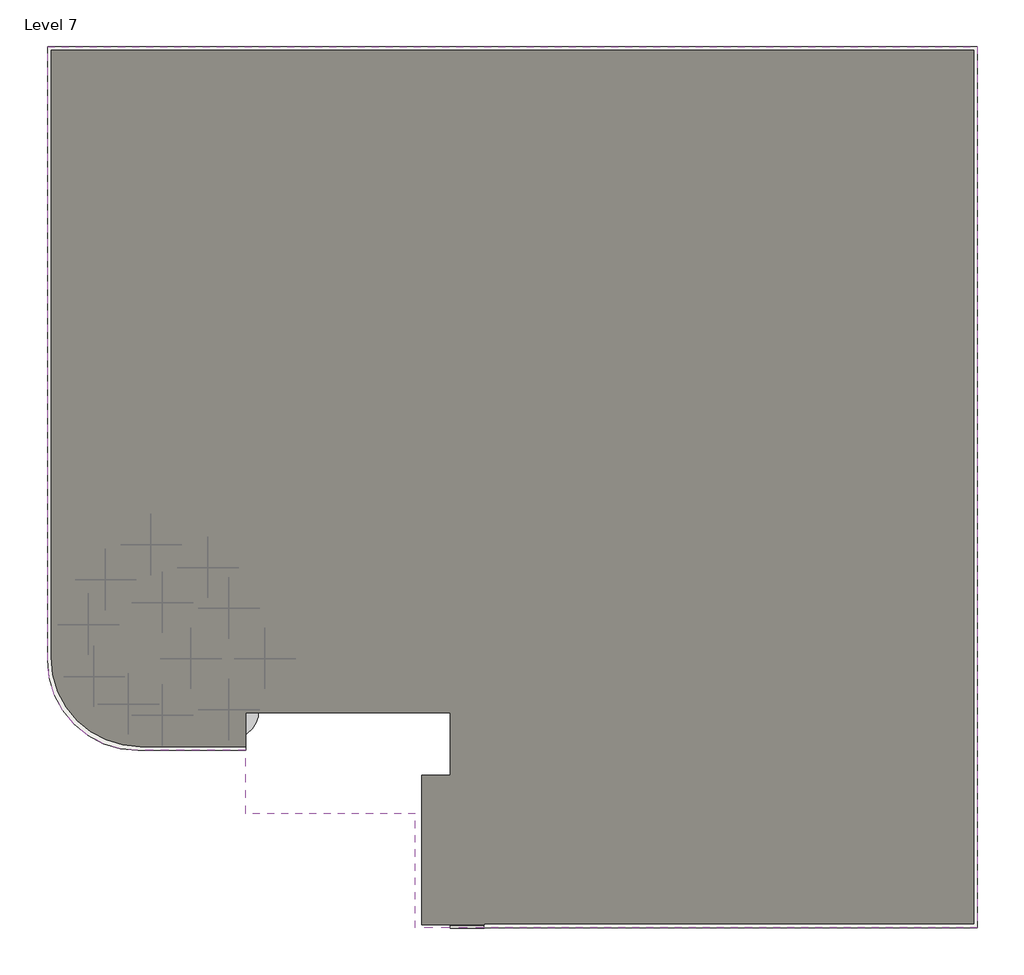
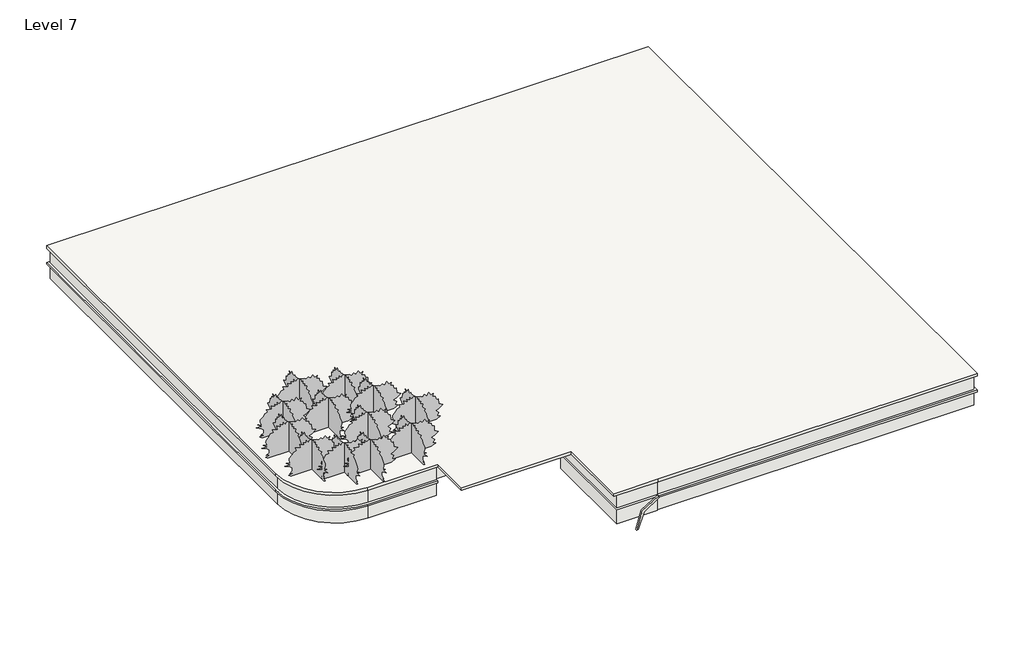
# One storey: 12 geographic elements, 4 slabs, 1 wall.
"""IFC4 building model written with IfcOpenShell, lengths in millimetres."""

from ifc_helpers import new_model, si_unit, point, frame, frame_2d, origin, place, context, project, spatial, polyline, circle_curve, trimmed, segment, composite_curve, outline, extrude, transform, mapped, element, save
from components import rpc_shrub_d2795376

model = new_model("IFC4")

# Units and contexts
model_context = context("Model", 3, world=origin())
ifc_project = project(units=[si_unit("LENGTHUNIT", "METRE", prefix="MILLI")], contexts=[model_context])

# Site, building, storey
site = spatial("IfcSite", under=ifc_project)
building = spatial("IfcBuilding", under=site)
storey = spatial("IfcBuildingStorey", under=building, Name="Level 7", Elevation=15240.0)

# Geographic elements
placement = place(None, origin())
rpc_shrub_shape = rpc_shrub_d2795376(model_context)
element("IfcGeographicElement", 1, ObjectType="RPC Shrub", at=placement, inside=storey, context=model_context, shape_type="MappedRepresentation", body=[
    mapped(rpc_shrub_shape, transform((-13877.236879, -1580.5602909, 16306.8), x_axis=(1.0, 0.0, 0.0), y_axis=(0.0, 1.0, 0.0), z_axis=(0.0, 0.0, 1.0))),
])
element("IfcGeographicElement", 2, ObjectType="RPC Shrub", at=placement, inside=storey, context=model_context, shape_type="MappedRepresentation", body=[
    mapped(rpc_shrub_shape, transform((-11896.036879, -1580.5602909, 16306.8), x_axis=(1.0, 0.0, 0.0), y_axis=(0.0, 1.0, 0.0), z_axis=(0.0, 0.0, 1.0))),
])
element("IfcGeographicElement", 3, ObjectType="RPC Shrub", at=placement, inside=storey, context=model_context, shape_type="MappedRepresentation", body=[
    mapped(rpc_shrub_shape, transform((-14639.236879, -3104.5602909, 16306.8), x_axis=(1.0, 0.0, 0.0), y_axis=(0.0, 1.0, 0.0), z_axis=(0.0, 0.0, 1.0))),
])
element("IfcGeographicElement", 4, ObjectType="RPC Shrub", at=placement, inside=storey, context=model_context, shape_type="MappedRepresentation", body=[
    mapped(rpc_shrub_shape, transform((-16163.236879, 529.4091958, 16306.8), x_axis=(1.0, 0.0, 0.0), y_axis=(0.0, 1.0, 0.0), z_axis=(0.0, 0.0, 1.0))),
])
element("IfcGeographicElement", 5, ObjectType="RPC Shrub", at=placement, inside=storey, context=model_context, shape_type="MappedRepresentation", body=[
    mapped(rpc_shrub_shape, transform((-14639.236879, -80.1908042, 16306.8), x_axis=(1.0, 0.0, 0.0), y_axis=(0.0, 1.0, 0.0), z_axis=(0.0, 0.0, 1.0))),
])
element("IfcGeographicElement", 6, ObjectType="RPC Shrub", at=placement, inside=storey, context=model_context, shape_type="MappedRepresentation", body=[
    mapped(rpc_shrub_shape, transform((-12861.236879, -2952.1602909, 16306.8), x_axis=(1.0, 0.0, 0.0), y_axis=(0.0, 1.0, 0.0), z_axis=(0.0, 0.0, 1.0))),
])
element("IfcGeographicElement", 7, ObjectType="RPC Shrub", at=placement, inside=storey, context=model_context, shape_type="MappedRepresentation", body=[
    mapped(rpc_shrub_shape, transform((-12861.236879, -232.5908042, 16306.8), x_axis=(1.0, 0.0, 0.0), y_axis=(0.0, 1.0, 0.0), z_axis=(0.0, 0.0, 1.0))),
])
element("IfcGeographicElement", 8, ObjectType="RPC Shrub", at=placement, inside=storey, context=model_context, shape_type="MappedRepresentation", body=[
    mapped(rpc_shrub_shape, transform((-16620.436879, -666.1602909, 16306.8), x_axis=(1.0, 0.0, 0.0), y_axis=(0.0, 1.0, 0.0), z_axis=(0.0, 0.0, 1.0))),
])
element("IfcGeographicElement", 9, ObjectType="RPC Shrub", at=placement, inside=storey, context=model_context, shape_type="MappedRepresentation", body=[
    mapped(rpc_shrub_shape, transform((-14944.036879, 1467.4397091, 16306.8), x_axis=(1.0, 0.0, 0.0), y_axis=(0.0, 1.0, 0.0), z_axis=(0.0, 0.0, 1.0))),
])
element("IfcGeographicElement", 10, ObjectType="RPC Shrub", at=placement, inside=storey, context=model_context, shape_type="MappedRepresentation", body=[
    mapped(rpc_shrub_shape, transform((-13420.036879, 857.8397091, 16306.8), x_axis=(1.0, 0.0, 0.0), y_axis=(0.0, 1.0, 0.0), z_axis=(0.0, 0.0, 1.0))),
])
element("IfcGeographicElement", 11, ObjectType="RPC Shrub", at=placement, inside=storey, context=model_context, shape_type="MappedRepresentation", body=[
    mapped(rpc_shrub_shape, transform((-16468.036879, -2061.3908042, 16306.8), x_axis=(1.0, 0.0, 0.0), y_axis=(0.0, 1.0, 0.0), z_axis=(0.0, 0.0, 1.0))),
])
element("IfcGeographicElement", 12, ObjectType="RPC Shrub", at=placement, inside=storey, context=model_context, shape_type="MappedRepresentation", body=[
    mapped(rpc_shrub_shape, transform((-15553.636879, -2799.7602909, 16306.8), x_axis=(1.0, 0.0, 0.0), y_axis=(0.0, 1.0, 0.0), z_axis=(0.0, 0.0, 1.0))),
])

# Slabs
element("IfcSlab", 13, ObjectType="Generic - 2'", at=placement, inside=storey, context=model_context, shape_type="SweptSolid", body=[
    extrude(outline(composite_curve([segment(polyline([(7112.0, -8690.7908042), (-6003.236879, -8690.7908042), (-6003.236879, -8716.1908042), (-7679.636879, -8716.1908042), (-7679.636879, -4704.7602909), (-7374.836879, -4704.7602909), (-6917.636879, -4704.7602909), (-6917.636879, -3028.3602909), (-12404.036879, -3028.3602909), (-12404.036879, -3940.9908042), (-15222.9504174, -3940.9908042)]), True, "CONTINUOUS"), segment(trimmed(circle_curve(frame_2d((-15222.9504174, -1548.7562261)), 2392.2345781), [point((-15222.9504174, -3940.9908042))], [point((-17615.1849955, -1548.7562261))], False, "CARTESIAN"), True, "CONTINUOUS"), segment(polyline([(-17615.1849955, -1548.7562261), (-17615.1849955, 14724.0625), (-6003.236879, 14724.0625), (7112.0, 14724.0625), (7112.0, -8690.7908042)]), True, "CONTINUOUS")], self_intersect=False)), frame((0.0, 0.0, 15163.8), z_axis=(0.0, 0.0, 1.0), x_axis=(1.0, 0.0, 0.0)), (0.0, 0.0, 1.0), 609.6),
])
element("IfcSlab", 14, ObjectType="Generic - 2'", at=placement, inside=storey, context=model_context, shape_type="SweptSolid", body=[
    extrude(outline(composite_curve([segment(polyline([(7112.0, -8690.7908042), (-6003.236879, -8690.7908042), (-6003.236879, -8716.1908042), (-7679.636879, -8716.1908042), (-7679.636879, -4704.7602909), (-7374.836879, -4704.7602909), (-6917.636879, -4704.7602909), (-6917.636879, -3028.3602909), (-12404.036879, -3028.3602909), (-12404.036879, -3940.9908042), (-15222.9504174, -3940.9908042)]), True, "CONTINUOUS"), segment(trimmed(circle_curve(frame_2d((-15222.9504174, -1548.7562261)), 2392.2345781), [point((-15222.9504174, -3940.9908042))], [point((-17615.1849955, -1548.7562261))], False, "CARTESIAN"), True, "CONTINUOUS"), segment(polyline([(-17615.1849955, -1548.7562261), (-17615.1849955, 14724.0625), (-6003.236879, 14724.0625), (7112.0, 14724.0625), (7112.0, -8690.7908042)]), True, "CONTINUOUS")], self_intersect=False)), frame((0.0, 0.0, 15849.6), z_axis=(0.0, 0.0, 1.0), x_axis=(1.0, 0.0, 0.0)), (0.0, 0.0, 1.0), 609.6),
])
element("IfcSlab", 15, ObjectType="Generic - 3\"", at=placement, inside=storey, context=model_context, shape_type="SweptSolid", body=[
    extrude(outline(composite_curve([segment(polyline([(-6003.236879, 14825.6625), (7213.6, 14825.6625), (7213.6, -8792.3908042), (-6003.236879, -8792.3908042), (-6003.236879, -2875.9602909), (-6892.236879, -2875.9602909), (-6915.8673923, -2899.5908042), (-12397.5833185, -2899.5908042), (-12397.5833185, -3051.9908042), (-12397.5833185, -4040.2121743), (-15293.1833185, -4040.2121743)]), True, "CONTINUOUS"), segment(trimmed(circle_curve(frame_2d((-15293.1833185, -1620.7586138)), 2419.4535605), [point((-15293.1833185, -4040.2121743))], [point((-17712.636879, -1620.7586138))], False, "CARTESIAN"), True, "CONTINUOUS"), segment(polyline([(-17712.636879, -1620.7586138), (-17712.636879, 14825.6625), (-6003.236879, 14825.6625)]), True, "CONTINUOUS")], self_intersect=False)), frame((0.0, 0.0, 15773.4), z_axis=(0.0, 0.0, 1.0), x_axis=(1.0, 0.0, 0.0)), (0.0, 0.0, 1.0), 76.2),
])
element("IfcSlab", 16, ObjectType="Generic - 5\"", at=placement, inside=storey, context=model_context, shape_type="SweptSolid", body=[
    extrude(outline(composite_curve([segment(polyline([(-6003.236879, 14825.6625), (7213.6, 14825.6625), (7213.6, -8792.3908042), (-6003.236879, -8792.3908042), (-7850.9833185, -8792.3908042), (-7850.9833185, -5740.4), (-12397.5833185, -5740.4), (-12397.5833185, -4040.2121743), (-15293.1833185, -4040.2121743)]), True, "CONTINUOUS"), segment(trimmed(circle_curve(frame_2d((-15293.1833185, -1620.7586138)), 2419.4535605), [point((-15293.1833185, -4040.2121743))], [point((-17712.636879, -1620.7586138))], False, "CARTESIAN"), True, "CONTINUOUS"), segment(polyline([(-17712.636879, -1620.7586138), (-17712.636879, 14825.6625), (-6003.236879, 14825.6625)]), True, "CONTINUOUS")], self_intersect=False)), frame((0.0, 0.0, 16459.2), z_axis=(0.0, 0.0, 1.0), x_axis=(1.0, 0.0, 0.0)), (0.0, 0.0, 1.0), 127.0),
])

# Wall
element("IfcWall", 17, ObjectType="Generic - 3\"", at=placement, inside=storey, context=model_context, shape_type="SweptSolid", body=[
    extrude(outline(composite_curve([segment(trimmed(circle_curve(frame_2d((14653.5847682, -5674.4463462)), 1167.0858442), [point((14668.5, -6841.436879))], [point((15773.4, -6003.236879))], True, "CARTESIAN"), True, "CONTINUOUS"), segment(polyline([(15773.4, -6003.236879), (15849.6, -6003.236879)]), True, "CONTINUOUS"), segment(trimmed(circle_curve(frame_2d((14714.7567548, -5757.3914372)), 1161.1671596), [point((15849.6, -6003.236879))], [point((14668.5, -6917.636879))], False, "CARTESIAN"), True, "CONTINUOUS"), segment(polyline([(14668.5, -6917.636879), (14668.5, -6841.436879)]), True, "CONTINUOUS")], self_intersect=False)), frame((0.0, -8811.4408042, 0.0), z_axis=(0.0, 1.0, 0.0), x_axis=(0.0, 0.0, 1.0)), (0.0, 0.0, 1.0), 76.2),
])

save(model, "model.ifc")

# Revit data of these elements
# Type "RPC Shrub"
#   built-in parameter 1005198 = "{2, 15},{39, RPC-16-G3GJ-A6PX-PK1P-U000-ST1L-LVER-AU},{1, 0},{1, 0},{2, 13},{1, 8},{5, Color},{1, 0},{1, 0},{3, 0.8},{3, 0.8},{3, 0.8},{1, 8},{7, BBoxMin},{1, 0},{1, 0},{1, 0},{1, 0},{1, 0},{1, 8},{7, BBoxMax},{1, 0},{1, 0},{1, 0},{1, 0},{1, 0},{2, 11},{9, RPCTypeId},{1, 0},{1, 0},{39, RPC-16-G3GJ-A6PX-PK1P-U000-ST1L-LVER-AU},{1, 6},{14, RPCPlantHeight},{1, 0},{1, 0},{7, 5.33333},{2, 11},{7, keyword},{1, 0},{1, 0},{35, :RPCs:Shrubs & Grasses:Geometry:RPC},{2, 11},{8, category},{1, 0},{1, 0},{16, Shrubs & Grasses},{2, 11},{12, LocalizedUID},{1, 0},{1, 0},{8, Oleander},{2, 14},{6, Height},{1, 0},{1, 0},{7, 5.33333},{1, 2},{16, Cast Reflections},{1, 0},{1, 0},{1, 0},{1, 2},{12, Cast Shadows},{1, 0},{1, 0},{1, 1},{1, 2},{9, Lock View},{1, 0},{1, 0},{1, 0},{1, 4},{5, ViewC},{1, 0},{1, 0},{1, 0},{21, assetlibrary_base.fbx},{1, 5},"
#   built-in parameter 1005195 = "RPC-16-G3GJ-A6PX-PK1P-U000-ST1L-LVER-AU"
#   Assembly Code = "G2050500"
#   Height = 5' - 4"
#   Default Elevation = 0
# Type "Generic - 2'"
#   Assembly Code = "B1010"
#   Function = 0
#   Layers, outside or top first: 2' - 0" "Parking Stripe" (function 1)
# Type "Generic - 3\""
#   Assembly Code = "B1010"
#   Function = 0
#   Layers, outside or top first: 0' - 3" "Rigid insulation" (function 1)
# Type "Generic - 5\""
#   Assembly Code = "B1010"
#   Function = 0
#   Layers, outside or top first: 0' - 5" "Rigid insulation" (function 1)
# Type "Generic - 3\""
#   Assembly Code = "B2010"
#   Layers, outside or top first: 0' - 3" "TV - Black" (function 1)
# Elements 1, 2, 3, 4, 5, 6, 7, 8, 9, 10, 11, 12 (IfcGeographicElement, "RPC Shrub")
#   Phase Created = New Construction
# Element 13 (IfcSlab, "Generic - 2'")
#   built-in parameter 1001955 = 3.14159 (stored number, unit not read)
#   Height Offset From Level = 1' - 9"
#   Phase Created = New Construction
#   Materials on its faces: "Parking Stripe", "Door - Frame"
# Element 14 (IfcSlab, "Generic - 2'")
#   built-in parameter 1001955 = 3.14159 (stored number, unit not read)
#   Height Offset From Level = 4' - 0"
#   Phase Created = New Construction
#   Materials on its faces: "Parking Stripe"
# Element 15 (IfcSlab, "Generic - 3\"")
#   built-in parameter 1001955 = 3.14159 (stored number, unit not read)
#   Height Offset From Level = 2' - 0"
#   Phase Created = New Construction
#   Materials on its faces: "Rigid insulation"
# Element 16 (IfcSlab, "Generic - 5\"")
#   built-in parameter 1001955 = 3.14159 (stored number, unit not read)
#   Height Offset From Level = 4' - 5"
#   Phase Created = New Construction
#   Materials on its faces: "Rigid insulation", "Steel, Paint Finish, Ivory, Glossy"
# Element 17 (IfcWall, "Generic - 3\"")
#   built-in parameter 1001111 = -1' - 10 1/2"
#   Top Offset = 0' - 0"
#   Base Offset = -1' - 10 1/2"
#   Unconnected Height = 4' - 6 1/2"
#   wall height = 4' - 6 1/2"
#   Phase Created = New Construction
#   Base Constraint = Level 7
#   Materials on its faces: "TV - Black"
# Materials
#   "Parking Stripe": class "Paint", colour RGB 250 250 91, transparency 0, Cost = 0
#   "Rigid insulation": class "Generic", colour RGB 127 127 127, transparency 0, Description = "Rigid foam insulation board", Cost = 0
#   "TV - Black": colour RGB 49 49 49, transparency 0
#   "Door - Frame": colour RGB 118 70 51, transparency 0, Cost = 0
#   "Steel, Paint Finish, Ivory, Glossy": class "Metal", colour RGB 247 247 239, transparency 0, Description = "Steel, paint finish, ivory, glossy", Cost = 0
